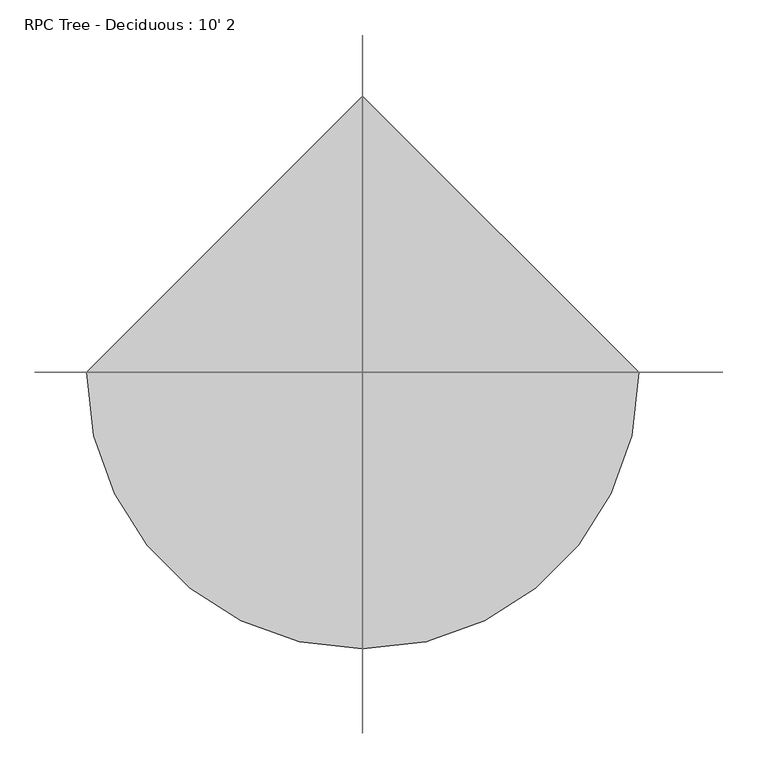
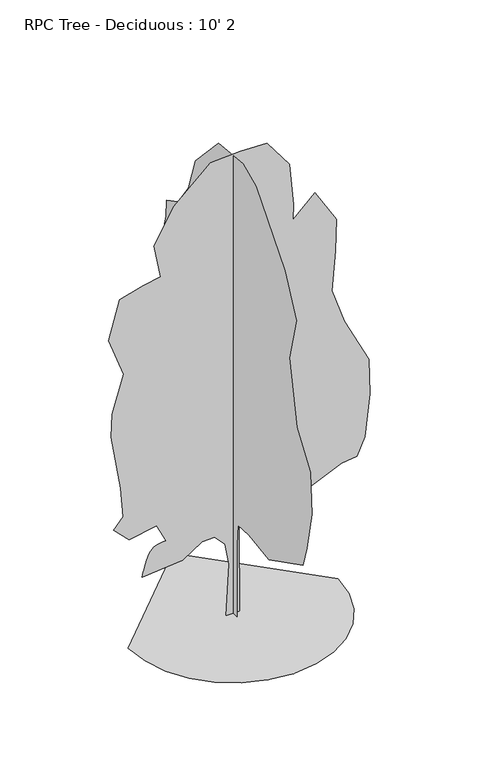
"""IFC4 building model written with IfcOpenShell, lengths in millimetres: geographic element geometry, RPC Tree - Deciduous : 10' 2."""

from ifc_helpers import new_model, si_unit, origin, place, context, project, spatial, triangles, source, transform, mapped, element, save


def rpc_tree_deciduous_10_2_5dd3353f(model_context):
    return source(origin(), model_context, "Body", "Tessellation", [
        triangles([(-657.9809858, 0.0, 2.47e-05), (-640.5860447, -150.7657429, 2.47e-05), (-591.0457546, -289.2199553, 2.47e-05), (-513.3265523, -411.3957464, 2.47e-05), (-411.3957828, -513.3266613, 2.47e-05), (-289.2198827, -591.0456093, 2.47e-05), (-150.7656703, -640.5860447, 2.47e-05), (2.88e-05, -657.9809858, 2.47e-05), (150.765752, -640.5861174, 2.47e-05), (289.2199735, -591.0457183, 2.47e-05), (411.3957828, -513.3265523, 2.47e-05), (513.326734, -411.3957828, 2.47e-05), (591.045682, -289.2198645, 2.47e-05), (640.5860447, -150.7656339, 2.47e-05), (657.9809858, 5.75e-05, 2.47e-05), (-8.63e-05, 657.9809858, 2.47e-05), (-4.3e-06, -41.1385046, 0.0), (1e-05, -40.4986863, 477.8216337), (1.29e-05, -51.9527836, 615.1211746), (3e-07, -175.5301652, 623.2661716), (-2.31e-05, -390.5565024, 591.3227726), (-5.62e-05, -761.4770668, 779.4708086), (-5.65e-05, -804.4823633, 919.2380768), (-5.44e-05, -858.2390385, 1177.2697105), (-4.47e-05, -842.1121885, 1446.0528683), (-2.32e-05, -696.1527838, 1656.406889), (-2.2e-06, -610.9594374, 2064.2539421), (-1.4e-06, -686.2180704, 2354.5395664), (1.92e-05, -562.5780155, 2612.5713455), (6.28e-05, -250.7897429, 2983.4920189), (7.94e-05, -109.2802846, 3047.2776604), (0.0001065, 157.7606466, 3021.1216988), (0.0001248, 410.4167364, 2752.3386864), (0.000126, 485.6760962, 2526.5608978), (0.0001329, 598.5645181, 2365.2909451), (0.0001439, 722.2052633, 2300.7831093), (0.0001413, 727.58088, 2193.269759), (0.0001409, 759.8349432, 2069.6296314), (0.000131, 706.0782681, 1924.4868919), (0.0001319, 754.4592539, 1784.7196964), (0.0001312, 802.840167, 1591.1958984), (0.0001284, 792.0889338, 1537.4391506), (0.0001151, 700.7027241, 1408.4231884), (0.0001092, 694.9245884, 1231.0264584), (0.0001053, 689.9512728, 1118.1374914), (0.0001017, 695.3269621, 978.3704412), (9.65e-05, 700.7027241, 784.8467159), (8.69e-05, 625.443437, 725.7142788), (7.23e-05, 485.6762778, 725.7142788), (7.31e-05, 550.1842226, 526.8148642), (6.86e-05, 539.398035, 413.9538025), (6.07e-05, 441.2124221, 491.1345566), (3.95e-05, 251.7850674, 442.6830445), (3.92e-05, 220.684731, 542.8243884), (2.51e-05, 86.3651045, 541.6010256), (2.01e-05, 52.3204937, 491.3338177), (1.31e-05, 31.8197329, 327.3132697), (4.7e-06, 44.8664066, 5.1e-06), (-44.3483468, 1.9e-06, 1.78e-05), (-26.6845903, -3.86e-05, 333.4006525), (-51.7229194, -5.44e-05, 475.1774274), (-116.3151477, -6e-05, 546.1270575), (-193.4545798, -5.63e-05, 543.4785273), (-318.5071212, -4.12e-05, 462.3069194), (-571.163211, -2.76e-05, 440.8043438), (-567.6682571, -2.94e-05, 454.7058572), (-563.9382159, -3.13e-05, 469.0775454), (-559.7379999, -3.33e-05, 484.3894741), (-554.8325217, -3.55e-05, 501.1121452), (-548.9867303, -3.8e-05, 519.7150795), (-541.9654655, -4.08e-05, 540.6693601), (-533.5336764, -4.4e-05, 564.444435), (-522.9077625, -4.71e-05, 586.4957053), (-509.7428321, -4.96e-05, 602.6226643), (-494.4621878, -5.16e-05, 613.8126789), (-477.4888052, -5.32e-05, 621.053516), (-459.246096, -5.45e-05, 625.3319613), (-440.1569269, -5.56e-05, 627.6358177), (-420.6446732, -5.66e-05, 628.9523798), (-479.7768559, -6.81e-05, 747.2169634), (-651.798151, -5.67e-05, 714.9629728), (-748.5599047, -6.4e-05, 811.7250172), (-689.4276129, -7.5e-05, 881.6086149), (-705.5546082, -9.73e-05, 1075.1324129), (-764.6868273, -0.0001377, 1435.3014896), (-759.3923103, -0.0001557, 1584.466222), (-687.9670189, -0.0001875, 1825.330299), (-780.8138952, -0.0002139, 2080.3808647), (-710.9301521, -0.0002464, 2327.6614105), (-565.7874853, -0.0002579, 2370.6666344), (-455.3653009, -0.000265, 2390.1449512), (-495.9039602, -0.0002891, 2607.1958015), (-372.2636147, -0.0003208, 2827.5980461), (-141.1101186, -0.0003559, 3037.248912), (47.037872, -0.0003654, 3048.0), (213.6834868, -0.000372, 3042.6241653), (353.4506641, -0.0003557, 2854.4763474), (379.1488412, -0.000324, 2579.0071152), (375.4587685, -0.0003118, 2477.9879906), (514.7204352, -0.0003333, 2607.1958015), (649.1120504, -0.0003129, 2386.793557), (643.7363611, -0.0002878, 2178.6037937), (619.7830267, -0.000256, 1920.2608418), (697.4929636, -0.0002323, 1693.3332687), (852.7056553, -0.0002027, 1387.6792511), (857.6541904, -0.0001754, 1157.1237745), (826.5087805, -0.0001412, 881.6084696), (778.1278673, -0.0001257, 768.7195753), (681.3658957, -0.0001201, 757.9682693), (493.2178596, -0.0001017, 671.9576763), (326.5722176, -8.03e-05, 553.6931291), (102.9906158, -8.2e-05, 649.8275591), (37.220348, -7.07e-05, 579.0538994), (41.6620963, -1.8e-06, 1.41e-05)], [[15, 16, 1], [14, 15, 1], [14, 1, 2], [13, 14, 2], [13, 2, 3], [13, 3, 4], [12, 13, 4], [11, 12, 4], [11, 4, 5], [11, 5, 6], [11, 6, 7], [11, 7, 8], [11, 8, 9], [11, 9, 10], [50, 51, 52], [57, 58, 17], [57, 17, 18], [56, 57, 18], [56, 18, 19], [55, 56, 19], [49, 50, 52], [52, 53, 54], [49, 52, 54], [35, 36, 37], [46, 47, 48], [46, 48, 49], [21, 22, 23], [20, 21, 23], [20, 23, 24], [20, 24, 25], [20, 25, 26], [19, 20, 26], [19, 26, 27], [45, 46, 49], [31, 32, 33], [30, 31, 33], [29, 30, 33], [29, 33, 34], [28, 29, 34], [27, 28, 34], [19, 27, 34], [19, 34, 35], [19, 35, 37], [19, 37, 38], [19, 38, 39], [19, 39, 40], [19, 40, 41], [19, 41, 42], [19, 42, 43], [19, 43, 44], [19, 44, 45], [19, 45, 49], [19, 49, 54], [55, 19, 54], [64, 65, 66], [64, 66, 67], [64, 67, 68], [99, 100, 101], [64, 68, 69], [64, 69, 70], [64, 70, 71], [114, 59, 60], [113, 114, 60], [113, 60, 61], [113, 61, 62], [64, 71, 72], [64, 72, 73], [64, 73, 74], [64, 74, 75], [64, 75, 76], [64, 76, 77], [64, 77, 78], [64, 78, 79], [63, 64, 79], [81, 82, 83], [80, 81, 83], [99, 101, 102], [107, 108, 109], [110, 111, 112], [88, 89, 90], [87, 88, 90], [87, 90, 91], [80, 83, 84], [95, 96, 97], [95, 97, 98], [94, 95, 98], [93, 94, 98], [92, 93, 98], [91, 92, 98], [91, 98, 99], [87, 91, 99], [87, 99, 102], [87, 102, 103], [87, 103, 104], [86, 87, 104], [85, 86, 104], [84, 85, 104], [80, 84, 104], [80, 104, 105], [80, 105, 106], [80, 106, 107], [80, 107, 109], [80, 109, 110], [80, 110, 112], [79, 80, 112], [63, 79, 112], [62, 63, 112], [113, 62, 112]], closed=False),
    ])


if __name__ == "__main__":
    model = new_model("IFC4")
    model_context = context("Model", 3, world=origin())
    ifc_project = project(units=[si_unit("LENGTHUNIT", "METRE", prefix="MILLI")], contexts=[model_context])
    site = spatial("IfcSite", under=ifc_project)
    building = spatial("IfcBuilding", under=site)
    placement = place(None, origin())
    rpc_tree_deciduous_10_2_shape = rpc_tree_deciduous_10_2_5dd3353f(model_context)
    element("IfcGeographicElement", 1, ObjectType="RPC Tree - Deciduous : 10' 2", at=placement, inside=building, context=model_context, shape_type="MappedRepresentation", body=[
        mapped(rpc_tree_deciduous_10_2_shape, transform((0.0, 0.0, 0.0), x_axis=(1.0, 0.0, 0.0), y_axis=(0.0, 1.0, 0.0), z_axis=(0.0, 0.0, 1.0))),
    ])
    save(model, "model.ifc")

# Revit data of these elements
# Type "RPC Tree - Deciduous : 10' 2"
#   built-in parameter 1005198 = "{2, 15},{22, RPC-8-G3GR-497X-PHW5-6},{1, 0},{1, 0},{2, 15},{1, 8},{5, Color},{1, 0},{1, 0},{3, 0.8},{3, 0.8},{3, 0.8},{1, 8},{7, BBoxMin},{1, 0},{1, 0},{1, 0},{1, 0},{1, 0},{1, 8},{7, BBoxMax},{1, 0},{1, 0},{1, 0},{1, 0},{1, 0},{2, 11},{9, RPCTypeId},{1, 0},{1, 0},{22, RPC-8-G3GR-497X-PHW5-6},{1, 6},{14, RPCPlantHeight},{1, 0},{1, 0},{2, 25},{2, 11},{7, keyword},{1, 0},{1, 0},{34, :RPCs:Trees [General]:Geometry:RPC},{2, 11},{8, category},{1, 0},{1, 0},{15, Trees [General]},{2, 11},{12, LocalizedUID},{1, 0},{1, 0},{7, Red Ash},{2, 14},{6, Height},{1, 0},{1, 0},{2, 25},{1, 2},{16, Cast Reflections},{1, 0},{1, 0},{1, 0},{1, 2},{6, Jitter},{1, 0},{1, 0},{1, 1},{1, 2},{9, Billboard},{1, 0},{1, 0},{1, 0},{1, 2},{12, Cast Shadows},{1, 0},{1, 0},{1, 1},{1, 2},{20, Apply Filter Effects},{1, 0},{1, 0},{1, 0},{2, 11},{28, Apply Filter Effects-Text-FC},{1, 0},{1, 0},{4, None},{21, assetlibrary_base.fbx},{1, 5},"
#   built-in parameter 1005195 = "RPC-8-G3GR-497X-PHW5-6"
#   Type Comments = "Red Maple"
#   Assembly Code = "G2050500"
#   Height = 10' - 0"
#   Default Elevation = 0
